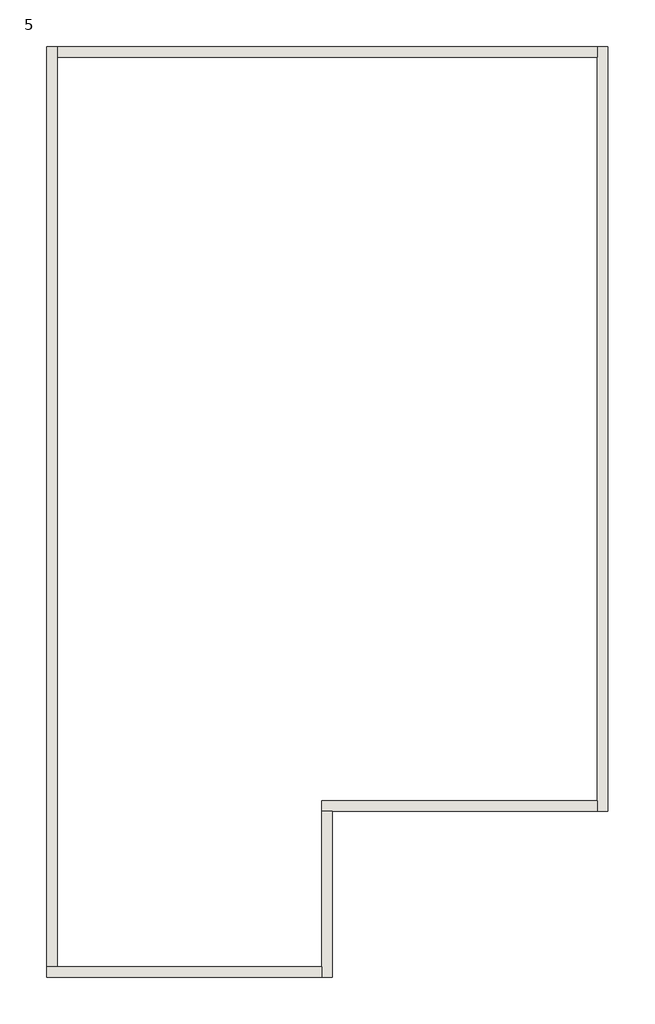
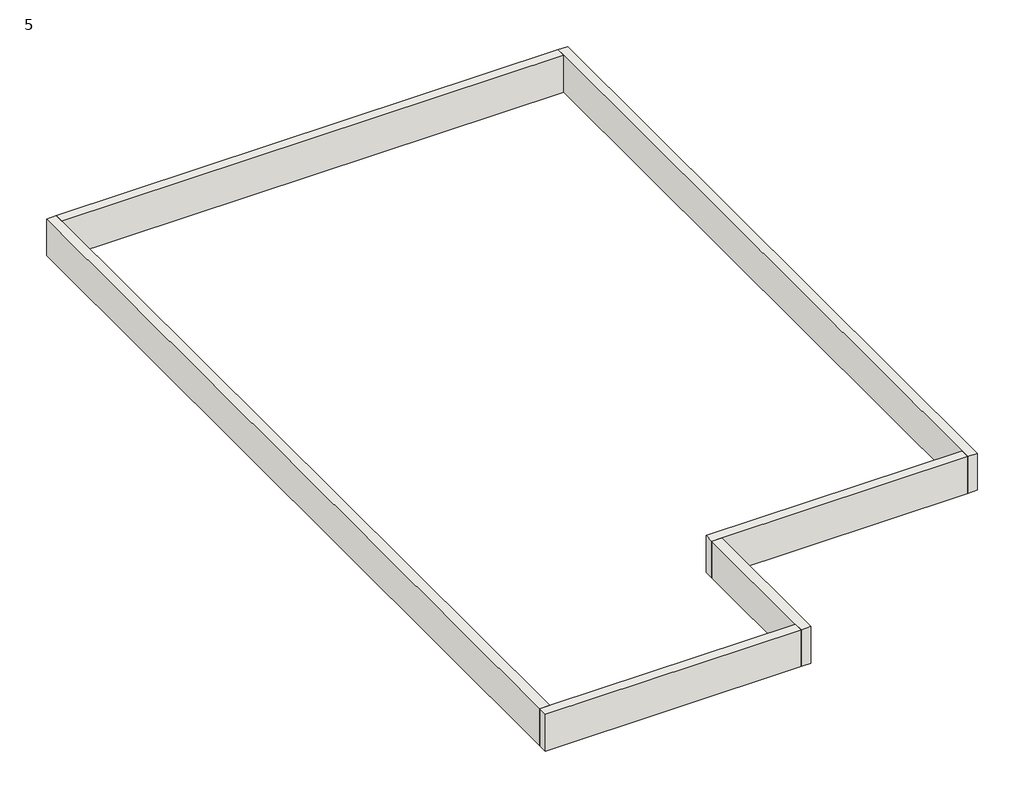
# One storey: 6 walls.
"""IFC4 building model written with IfcOpenShell, lengths in millimetres."""

from ifc_helpers import new_model, si_unit, frame, origin, place, context, project, spatial, polyline, outline, extrude, faceted_brep, element, save

model = new_model("IFC4")

# Units and contexts
model_context = context("Model", 3, world=origin())
ifc_project = project(units=[si_unit("LENGTHUNIT", "METRE", prefix="MILLI")], contexts=[model_context])

# Site, building, storey
site = spatial("IfcSite", under=ifc_project)
building = spatial("IfcBuilding", under=site)
storey = spatial("IfcBuildingStorey", under=building, Name="5", Elevation=7700.0)

# Walls
placement = place(None, origin())
element("IfcWall", 1, ObjectType="9\" wall", at=placement, inside=storey, context=model_context, shape_type="Brep", body=[
    faceted_brep([(5669.1463749, 10590.826913, 7700.0), (5669.1463749, 10362.226913, 7700.0), (5669.1463749, -5848.573087, 7700.0), (5669.1463749, -6077.173087, 7700.0), (5669.1463749, -6077.173087, 8614.4), (5669.1463749, -5848.573087, 8614.4), (5669.1463749, 10362.226913, 8614.4), (5669.1463749, 10590.826913, 8614.4), (5897.7463749, 10590.826913, 7700.0), (5897.7463749, 10590.826913, 8614.4), (5897.7463749, -6077.173087, 8614.4), (5897.7463749, -6077.173087, 7700.0)], [[[0, 1, 2, 3, 4, 5, 6, 7]], [[8, 9, 10, 11]], [[3, 2, 1, 0, 8, 11]], [[7, 6, 5, 4, 10, 9]], [[4, 3, 11, 10]], [[0, 7, 9, 8]]]),
])
element("IfcWall", 2, ObjectType="9\" wall", at=placement, inside=storey, context=model_context, shape_type="Brep", body=[
    faceted_brep([(5669.1463749, -5848.573087, 7700.0), (-338.0536251, -5848.573087, 7700.0), (-338.0536251, -5848.573087, 8614.4), (5669.1463749, -5848.573087, 8614.4), (5669.1463749, -6077.173087, 7700.0), (5669.1463749, -6077.173087, 8614.4), (-109.4536251, -6077.173087, 8614.4), (-338.0536251, -6077.173087, 8614.4), (-338.0536251, -6077.173087, 7700.0), (-109.4536251, -6077.173087, 7700.0)], [[[0, 1, 2, 3]], [[4, 5, 6, 7, 8, 9]], [[1, 0, 4, 9, 8]], [[3, 2, 7, 6, 5]], [[0, 3, 5, 4]], [[2, 1, 8, 7]]]),
])
element("IfcWall", 3, ObjectType="9\" wall", at=placement, inside=storey, context=model_context, shape_type="Brep", body=[
    faceted_brep([(-338.0536251, -6077.173087, 7700.0), (-338.0536251, -9474.973087, 7700.0), (-338.0536251, -9703.573087, 7700.0), (-338.0536251, -9703.573087, 8614.4), (-338.0536251, -9474.973087, 8614.4), (-338.0536251, -6077.173087, 8614.4), (-109.4536251, -6077.173087, 7700.0), (-109.4536251, -6077.173087, 8614.4), (-109.4536251, -9703.573087, 8614.4), (-109.4536251, -9703.573087, 7700.0)], [[[0, 1, 2, 3, 4, 5]], [[6, 7, 8, 9]], [[2, 1, 0, 6, 9]], [[5, 4, 3, 8, 7]], [[0, 5, 7, 6]], [[3, 2, 9, 8]]]),
])
element("IfcWall", 4, ObjectType="9\" wall", at=placement, inside=storey, context=model_context, shape_type="Brep", body=[
    faceted_brep([(-338.0536251, -9474.973087, 7700.0), (-6113.0536251, -9474.973087, 7700.0), (-6341.6536251, -9474.973087, 7700.0), (-6341.6536251, -9474.973087, 8614.4), (-6113.0536251, -9474.973087, 8614.4), (-338.0536251, -9474.973087, 8614.4), (-338.0536251, -9703.573087, 7700.0), (-338.0536251, -9703.573087, 8614.4), (-6341.6536251, -9703.573087, 8614.4), (-6341.6536251, -9703.573087, 7700.0)], [[[0, 1, 2, 3, 4, 5]], [[6, 7, 8, 9]], [[2, 1, 0, 6, 9]], [[5, 4, 3, 8, 7]], [[0, 5, 7, 6]], [[3, 2, 9, 8]]]),
])
element("IfcWall", 5, ObjectType="9\" wall", at=placement, inside=storey, context=model_context, shape_type="Brep", body=[
    faceted_brep([(-6113.0536251, -9474.973087, 7700.0), (-6113.0536251, 10362.226913, 7700.0), (-6113.0536251, 10590.826913, 7700.0), (-6113.0536251, 10590.826913, 8614.4), (-6113.0536251, 10362.226913, 8614.4), (-6113.0536251, -9474.973087, 8614.4), (-6341.6536251, -9474.973087, 7700.0), (-6341.6536251, -9474.973087, 8614.4), (-6341.6536251, 10590.826913, 8614.4), (-6341.6536251, 10590.826913, 7700.0)], [[[0, 1, 2, 3, 4, 5]], [[6, 7, 8, 9]], [[2, 1, 0, 6, 9]], [[5, 4, 3, 8, 7]], [[0, 5, 7, 6]], [[3, 2, 9, 8]]]),
])
element("IfcWall", 6, ObjectType="9\" wall", at=placement, inside=storey, context=model_context, shape_type="SweptSolid", body=[
    extrude(outline(polyline([(5669.1463749, 10362.226913), (-6113.0536251, 10362.226913), (-6113.0536251, 10590.826913), (5669.1463749, 10590.826913), (5669.1463749, 10362.226913)])), frame((0.0, 0.0, 7700.0), z_axis=(0.0, 0.0, 1.0), x_axis=(1.0, 0.0, 0.0)), (0.0, 0.0, 1.0), 914.4),
])

save(model, "model.ifc")

# Revit data of these elements
# Type "9\" wall"
#   Assembly Code = "B2010"
#   Layers, outside or top first: 0' - 9" "Laminate, Ivory, Matte" (function 1)
# Elements 1, 2, 3, 4, 5, 6 (IfcWall, "9\" wall")
#   Top Offset = 0' - 0"
#   Base Offset = 0' - 0"
#   wall height = 3' - 0"
#   Phase Created = New Construction
#   Base Constraint = 5
#   Top Constraint = 6
#   Materials on its faces: "Laminate, Ivory, Matte"
# Materials
#   "Laminate, Ivory, Matte": class "Plastic", colour RGB 247 247 239, transparency 0, Description = "Plastic Laminate - Ivory, Matte", Cost = 0
